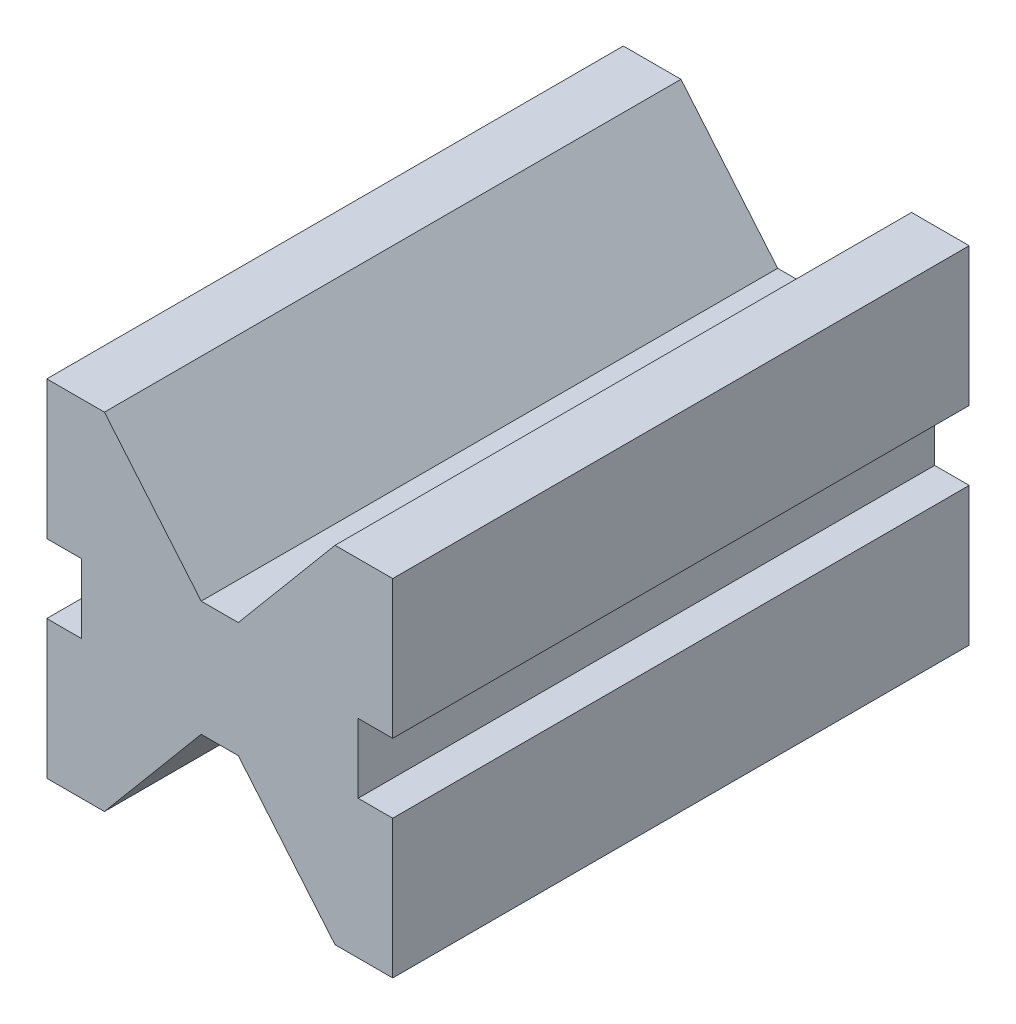
from build123d import *

# Parameters (mm, degrees)
V_BLOCK_BODY_EXTRUDE_100_DEPTH = 100


with BuildPart() as part:
    # V-Block Profile Sketch → V-Block Body Extrude 100 (new body)
    with BuildSketch(Plane.XY):
        Polygon((-30, -6), (-30, -30), (-20, -30), (-3.218007376, -10), (0, -10), (3.218007376, -10), (20, -30), (30, -30), (30, -6), (24, -6), (24, 6), (30, 6), (30, 30), (20, 30), (3.218007376, 10), (0, 10), (-3.218007376, 10), (-20, 30), (-30, 30), (-30, 6), (-24, 6), (-24, -6), align=None)
    extrude(amount=-V_BLOCK_BODY_EXTRUDE_100_DEPTH)


solid = part.part
